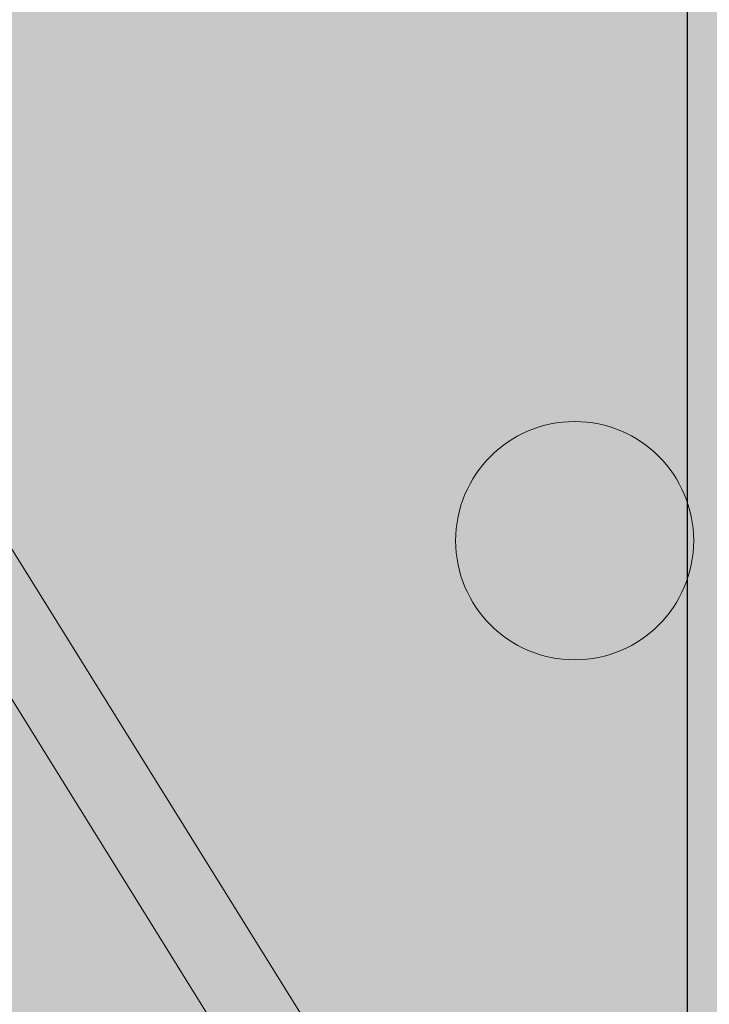
# Model space of a CAD drawing. Units: millimetres. Extents: x 11032 to 26788, y 3406 to 24505.
# Tile 52 of 78: x 15924 to 16358, y 15746 to 16366. Entities that reach past the tile are written whole.
import ezdxf

# ---------------------------------------------------------------- set-up
doc = ezdxf.new("R2010")
doc.units = ezdxf.units.MM
doc.header["$MEASUREMENT"] = 0
for name, color, linetype, lineweight in [('A-ANNO-DIMS', 2, 'Continuous', 18), ('A-GLAZ', 250, 'Continuous', 20), ('A-ROOF', 7, 'Continuous', 30), ('E-LITE', 7, 'Continuous', 18), ('E-LITE-PATT', 7, 'Continuous', 13)]:
    doc.layers.add(name, color=color, linetype=linetype, lineweight=lineweight)
doc.layers.add('A-GLAZ-FRAM-PATT', color=250, linetype='Continuous', lineweight=13, true_color=0x262627)
doc.layers.add('A-ROOF-PATT', color=9, linetype='Continuous', lineweight=13, true_color=0xc7c8ca)
doc.styles.get("Standard").update_dxf_attribs({"font": 'arial.ttf'})
doc.dimstyles.get("Standard").update_dxf_attribs({"dimtxt": 150, "dimasz": 100, "dimexe": 10, "dimexo": 5, "dimgap": 5, "dimtad": 0, "dimtih": 1, "dimtoh": 1, "dimdec": 0, "dimzin": 0, "dimdsep": 46, "dimtxsty": 'Standard', "dimcen": 0.09, "dimadec": 0, "dimazin": 0, "dimtfac": 1, "dimtdec": 0, "dimtofl": 0, "dimtmove": 0, "dimatfit": 3, "dimfxl": 1, "dimtolj": 1, "dimtzin": 0, "dimarcsym": 0})

# ---------------------------------------------------------------- blocks, each defined once
blk = doc.blocks.new('RECESSED-LIGHT-150')
blk.add_circle((75, 75), 75)
blk = doc.blocks.new('*D36')
at = {"layer": 'A-ANNO-DIMS', "color": 0, "lineweight": -2, "transparency": 16777216}
for p, q in [((12301.26, 17115.89), (12301.26, 24416.86)), ((25397.4, 4466.4), (25397.4, 24416.86)), ((12401.26, 24406.86), (18569.2, 24406.86)), ((25297.4, 24406.86), (19129.47, 24406.86))]:
    blk.add_line(p, q, dxfattribs=at)
at = {"layer": 'A-ANNO-DIMS', "color": 0, "transparency": 16777216}
for points in [[(12401.26, 24423.52), (12401.26, 24390.19), (12301.26, 24406.86)], [(25297.4, 24423.52), (25297.4, 24390.19), (25397.4, 24406.86)]]:
    blk.add_solid(points, dxfattribs=at)
at = {"layer": 'Defpoints', "color": 0, "transparency": 16777216}
for p in [(25397.4, 24406.86), (12301.26, 17110.89), (25397.4, 4461.4)]:
    blk.add_point(p, dxfattribs=at)
at = {"layer": 'A-ANNO-DIMS', "color": 0, "transparency": 16777216, "insert": (18849.33, 24406.86), "char_height": 150, "attachment_point": 5}
blk.add_mtext('\\A1;13096', dxfattribs=at)
blk = doc.blocks.new('*D37')
at = {"layer": 'A-ANNO-DIMS', "color": 0, "lineweight": -2, "transparency": 16777216}
for p, q in [((18087.74, 23450.36), (11334.76, 23450.36)), ((11344.76, 23350.36), (11344.76, 14037.46)), ((11344.76, 4561.4), (11344.76, 13874.29)), ((12927.66, 4461.4), (11334.76, 4461.4))]:
    blk.add_line(p, q, dxfattribs=at)
at = {"layer": 'A-ANNO-DIMS', "color": 0, "transparency": 16777216}
for points in [[(11328.1, 23350.36), (11361.43, 23350.36), (11344.76, 23450.36)], [(11328.1, 4561.4), (11361.43, 4561.4), (11344.76, 4461.4)]]:
    blk.add_solid(points, dxfattribs=at)
at = {"layer": 'Defpoints', "color": 0, "transparency": 16777216}
for p in [(11344.76, 23450.36), (18092.74, 23450.36), (12932.66, 4461.4)]:
    blk.add_point(p, dxfattribs=at)
at = {"layer": 'A-ANNO-DIMS', "color": 0, "transparency": 16777216, "insert": (11344.76, 13955.88), "char_height": 150, "attachment_point": 5}
blk.add_mtext('\\A1;18989', dxfattribs=at)
blk = doc.blocks.new('*D45')
at = {"layer": 'A-ANNO-DIMS', "color": 0, "lineweight": -2, "transparency": 16777216}
for p, q in [((13792.37, 18518.92), (26363.9, 18518.92)), ((26353.9, 18418.92), (26353.9, 17450.32)), ((26353.9, 16318.44), (26353.9, 17287.05)), ((22902.4, 16218.44), (26363.9, 16218.44))]:
    blk.add_line(p, q, dxfattribs=at)
at = {"layer": 'A-ANNO-DIMS', "color": 0, "transparency": 16777216}
for points in [[(26337.24, 18418.92), (26370.57, 18418.92), (26353.9, 18518.92)], [(26337.24, 16318.44), (26370.57, 16318.44), (26353.9, 16218.44)]]:
    blk.add_solid(points, dxfattribs=at)
at = {"layer": 'Defpoints', "color": 0, "transparency": 16777216}
for p in [(13787.37, 18518.92), (26353.9, 18518.92), (22897.4, 16218.44)]:
    blk.add_point(p, dxfattribs=at)
at = {"layer": 'A-ANNO-DIMS', "color": 0, "transparency": 16777216, "insert": (26353.9, 17368.68), "char_height": 150, "attachment_point": 5}
blk.add_mtext('\\A1;2300.5', dxfattribs=at)
blk = doc.blocks.new('*D57')
at = {"layer": 'A-ANNO-DIMS', "color": 0, "lineweight": -2, "transparency": 16777216}
for p, q in [((14994.7, 7266.4), (14994.7, 24416.86)), ((20894.7, 7266.4), (20894.7, 24416.86)), ((15094.7, 24406.86), (17715.98, 24406.86)), ((20794.7, 24406.86), (18173.42, 24406.86))]:
    blk.add_line(p, q, dxfattribs=at)
at = {"layer": 'A-ANNO-DIMS', "color": 0, "transparency": 16777216}
for points in [[(15094.7, 24423.52), (15094.7, 24390.19), (14994.7, 24406.86)], [(20794.7, 24423.52), (20794.7, 24390.19), (20894.7, 24406.86)]]:
    blk.add_solid(points, dxfattribs=at)
at = {"layer": 'Defpoints', "color": 0, "transparency": 16777216}
for p in [(20894.7, 24406.86), (14994.7, 7261.4), (20894.7, 7261.4)]:
    blk.add_point(p, dxfattribs=at)
at = {"layer": 'A-ANNO-DIMS', "color": 0, "transparency": 16777216, "insert": (17944.7, 24406.86), "char_height": 150, "attachment_point": 5}
blk.add_mtext('\\A1;5900', dxfattribs=at)
blk = doc.blocks.new('*D60')
at = {"layer": 'A-ANNO-DIMS', "color": 0, "lineweight": -2, "transparency": 16777216}
for p, q in [((14994.7, 7266.4), (14994.7, 24416.86)), ((16344.7, 7266.4), (16344.7, 24416.86)), ((15094.7, 24406.86), (15448.04, 24406.86)), ((16244.7, 24406.86), (15891.36, 24406.86))]:
    blk.add_line(p, q, dxfattribs=at)
at = {"layer": 'A-ANNO-DIMS', "color": 0, "transparency": 16777216}
for points in [[(15094.7, 24423.52), (15094.7, 24390.19), (14994.7, 24406.86)], [(16244.7, 24423.52), (16244.7, 24390.19), (16344.7, 24406.86)]]:
    blk.add_solid(points, dxfattribs=at)
at = {"layer": 'Defpoints', "color": 0, "transparency": 16777216}
for p in [(16344.7, 24406.86), (14994.7, 7261.4), (16344.7, 7261.4)]:
    blk.add_point(p, dxfattribs=at)
at = {"layer": 'A-ANNO-DIMS', "color": 0, "transparency": 16777216, "insert": (15669.7, 24406.86), "char_height": 150, "attachment_point": 5}
blk.add_mtext('\\A1;1350', dxfattribs=at)

msp = doc.modelspace()

# ---------------------------------------------------------------- hatches: boundary and pattern name
at = {"layer": 'A-GLAZ-FRAM-PATT'}
h = msp.add_hatch(color=256, dxfattribs=at)
edge = h.paths.add_edge_path()
edge.add_line((15784.393, 16248.213), (15784.393, 16153.61))
edge.add_line((15784.393, 16153.61), (16560.042, 14907.752))
edge.add_spline(control_points=[(16560.042, 14907.752), (16569.192, 14907.664), (16578.343, 14907.575), (16587.493, 14907.486), (16598.103, 14907.383), (16608.713, 14907.281), (16619.296, 14907.181)], knot_values=[1012.2878735, 1012.2878735, 1012.2878735, 1012.2878735, 1027.155312, 1027.155312, 1027.155312, 1044.3939449, 1044.3939449, 1044.3939449, 1044.3939449], degree=3, periodic=0)
edge.add_line((16619.296, 14907.181), (15784.393, 16248.213))
at = {"layer": 'A-ROOF-PATT'}
h = msp.add_hatch(color=256, dxfattribs=at)
edge = h.paths.add_edge_path()
edge.add_spline(control_points=[(17532.827, 17324.837), (17391.335, 17349.016), (16840.872, 17494.912), (16080.055, 18069.544), (14738.803, 18299.641), (13382.429, 18838.336), (12580.532, 17870.207), (12430.422, 17563.822)], knot_values=[2977.6027945, 2977.6027945, 2977.6027945, 2977.6027945, 3438.1840601, 4811.6463022, 5622.8675483, 7588.0288188, 8560.6685791, 8560.6685791, 8560.6685791, 8560.6685791], degree=3, periodic=0)
edge.add_spline(control_points=[(12430.422, 17563.822), (12437.904, 17573.36), (12445.386, 17582.899), (12452.869, 17592.437), (12452.869, 17592.438), (12452.869, 17592.438), (12452.869, 17592.438)], knot_values=[1408.564138, 1408.564138, 1408.564138, 1408.564138, 1444.85989, 1444.85989, 1444.85989, 1444.8601183, 1444.8601183, 1444.8601183, 1444.8601183], degree=3, periodic=0)
edge.add_spline(control_points=[(12452.869, 17592.438), (12555.432, 17723.185), (12736.557, 17929.686), (13044.86, 18114.643), (13219.943, 18189.644), (13299.92, 18220.646)], knot_values=[339.318246, 339.318246, 339.318246, 339.318246, 836.8349967, 1151.2512933, 1408.564138, 1408.564138, 1408.564138, 1408.564138], degree=3, periodic=0)
edge.add_spline(control_points=[(13299.92, 18220.646), (13299.998, 18220.689), (13300.077, 18220.732), (13319.738, 18231.488), (13339.24, 18241.402), (13388.645, 18264.703), (13418.466, 18277.069), (13478.019, 18298.648), (13507.751, 18307.861), (13544.561, 18317.488), (13551.584, 18319.245), (13558.612, 18320.924)], knot_values=[3783.8950972, 3783.8950972, 3783.8950972, 3783.8950972, 3784.1737101, 3784.1737101, 3853.4666747, 3853.4666747, 3960.2401917, 3960.2401917, 4067.0137087, 4067.0137087, 4092.1744649, 4092.1744649, 4092.1744649, 4092.1744649], degree=3, periodic=0)
edge.add_spline(control_points=[(13558.612, 18320.924), (13581.407, 18326.373), (13604.25, 18331.007), (13657.184, 18339.957), (13687.338, 18343.732), (13748.098, 18348.892), (13778.704, 18350.276), (13840.46, 18350.833), (13871.609, 18350.005), (13934.496, 18346.313), (13966.232, 18343.449), (14030.297, 18335.871), (14062.625, 18331.158), (14127.853, 18320.088), (14160.753, 18313.73), (14241.357, 18296.556), (14289.343, 18284.997), (14386.31, 18259.688), (14435.291, 18245.941), (14534.161, 18217.034), (14584.049, 18201.875), (14684.682, 18170.964), (14735.427, 18155.212), (14837.763, 18123.971), (14889.354, 18108.482), (14954.971, 18089.677), (14968.586, 18085.823), (14992.391, 18079.184), (15002.566, 18076.376), (15021.739, 18071.153), (15030.731, 18068.729), (15047.707, 18064.21), (15055.694, 18062.106), (15079.815, 18055.825), (15095.905, 18051.728), (15143.966, 18039.717), (15175.729, 18032.084), (15254.84, 18013.501), (15301.798, 18002.866), (15394.186, 17981.845), (15439.615, 17971.459), (15528.833, 17950.135), (15572.62, 17939.197), (15658.477, 17916.021), (15700.546, 17903.785), (15753.633, 17886.734), (15765.446, 17882.835), (15786.574, 17875.653), (15795.915, 17872.404), (15810.108, 17867.349), (15814.99, 17865.588), (15824.736, 17862.029), (15829.611, 17860.226), (15844.241, 17854.75), (15854.002, 17851.008), (15883.312, 17839.521), (15902.885, 17831.512), (15966.355, 17804.548), (16010.39, 17784.302), (16098.838, 17741.267), (16143.25, 17718.478), (16232.497, 17671.098), (16277.332, 17646.507), (16367.515, 17596.295), (16412.862, 17570.676), (16504.202, 17519.209), (16550.194, 17493.362), (16643.009, 17442.263), (16689.831, 17417.011), (16756.517, 17382.472), (16775.937, 17372.58), (16795.455, 17362.84)], knot_values=[4092.1744649, 4092.1744649, 4092.1744649, 4092.1744649, 4173.7872258, 4173.7872258, 4280.5607428, 4280.5607428, 4387.3342598, 4387.3342598, 4494.1077768, 4494.1077768, 4600.8812939, 4600.8812939, 4707.6548109, 4707.6548109, 4814.4283279, 4814.4283279, 4967.1262405, 4967.1262405, 5119.8241531, 5119.8241531, 5272.5220657, 5272.5220657, 5425.2199783, 5425.2199783, 5577.9178908, 5577.9178908, 5617.7853319, 5617.7853319, 5647.4648479, 5647.4648479, 5673.611025, 5673.611025, 5696.747607, 5696.747607, 5743.6818903, 5743.6818903, 5837.5504571, 5837.5504571, 5979.7261046, 5979.7261046, 6121.9017521, 6121.9017521, 6264.0773996, 6264.0773996, 6406.2530471, 6406.2530471, 6447.2585849, 6447.2585849, 6480.0420882, 6480.0420882, 6497.3077062, 6497.3077062, 6514.5733242, 6514.5733242, 6549.1045602, 6549.1045602, 6618.1670322, 6618.1670322, 6772.6610171, 6772.6610171, 6927.155002, 6927.155002, 7081.6489869, 7081.6489869, 7236.1429718, 7236.1429718, 7390.6369567, 7390.6369567, 7545.1309416, 7545.1309416, 7608.1992868, 7608.1992868, 7608.1992868, 7608.1992868], degree=3, periodic=0)
edge.add_spline(control_points=[(16795.455, 17362.84), (16814.335, 17349.456), (16832.897, 17336.263), (16873.225, 17307.197), (16894.778, 17291.386), (16936.221, 17259.941), (16956.11, 17244.308), (16993.863, 17213.094), (17011.726, 17197.514), (17041.993, 17169.265), (17054.791, 17156.601), (17078.762, 17131.225), (17089.933, 17118.516), (17110.618, 17092.991), (17120.131, 17080.178), (17130.17, 17065.264), (17131.487, 17063.277), (17133.77, 17059.776), (17134.746, 17058.261), (17136.69, 17055.205), (17137.657, 17053.668), (17140.539, 17049.025), (17142.438, 17045.89), (17148.068, 17036.367), (17151.732, 17029.859), (17163.03, 17008.788), (17170.335, 16993.646), (17184.087, 16961.978), (17190.534, 16945.453), (17202.562, 16911.165), (17208.142, 16893.402), (17218.448, 16856.821), (17223.173, 16838.003), (17231.801, 16799.51), (17235.705, 16779.837), (17241.533, 16746.739), (17243.676, 16733.5), (17247.718, 16706.37), (17249.608, 16692.472), (17252.066, 16672.69), (17252.761, 16666.875), (17254.1, 16655.226), (17254.744, 16649.4), (17256.596, 16631.917), (17257.727, 16620.254), (17260.823, 16585.238), (17262.489, 16561.858), (17266.551, 16488.654), (17267.658, 16438.661), (17267.349, 16375.228), (17267.193, 16362.07), (17266.95, 16348.891)], knot_values=[15.1130472, 15.1130472, 15.1130472, 15.1130472, 82.6995146, 82.6995146, 165.3990291, 165.3990291, 248.0985437, 248.0985437, 330.7980583, 330.7980583, 397.9419458, 397.9419458, 465.0858333, 465.0858333, 532.2297209, 532.2297209, 542.533741, 542.533741, 550.3568158, 550.3568158, 558.1798906, 558.1798906, 573.8260402, 573.8260402, 605.1183395, 605.1183395, 672.7640614, 672.7640614, 740.4097834, 740.4097834, 808.0555054, 808.0555054, 875.7012273, 875.7012273, 943.3469493, 943.3469493, 987.6613492, 987.6613492, 1033.4121612, 1033.4121612, 1052.3850876, 1052.3850876, 1071.358014, 1071.358014, 1109.3038668, 1109.3038668, 1185.1955724, 1185.1955724, 1346.4419026, 1346.4419026, 1388.5586631, 1388.5586631, 1388.5586631, 1388.5586631], degree=3, periodic=0)
edge.add_spline(control_points=[(17266.95, 16348.891), (17266.95, 16348.891), (17266.95, 16348.891), (17266.95, 16348.891), (17253.182, 15602.417), (17239.414, 14855.943), (17225.646, 14109.469)], knot_values=[1388.5586631, 1388.5586631, 1388.5586631, 1388.5586631, 1388.5589654, 1388.5589654, 1388.5589654, 3774.0767661, 3774.0767661, 3774.0767661, 3774.0767661], degree=3, periodic=0)
edge.add_spline(control_points=[(17225.646, 14109.469), (17226.198, 14109.827), (17226.748, 14110.185), (17242.065, 14120.191), (17255.956, 14130.116), (17274.422, 14144.286), (17279.609, 14148.386), (17284.686, 14152.511)], knot_values=[1926.3423968, 1926.3423968, 1926.3423968, 1926.3423968, 1927.316729, 1927.316729, 1953.5121761, 1953.5121761, 1964.0732348, 1964.0732348, 1964.0732348, 1964.0732348], degree=3, periodic=0)
edge.add_spline(control_points=[(17284.686, 14152.511), (17315.791, 14194.761), (17384.413, 14446.273), (17407.128, 14793.401), (17407.093, 15295.84), (17423.274, 15626.362), (17415.601, 15782.507)], knot_values=[0, 0, 0, 0, 163.2554674, 619.2296767, 1171.8624483, 1621.6355562, 1621.6355562, 1621.6355562, 1621.6355562], degree=3, periodic=0)
edge.add_spline(control_points=[(17415.601, 15782.507), (17438.21, 16077.57), (17410.495, 16533.484), (17390.893, 17030.649), (17301.082, 17169.349)], knot_values=[543.9784753, 543.9784753, 543.9784753, 543.9784753, 1452.9852767, 1960.0114926, 1960.0114926, 1960.0114926, 1960.0114926], degree=3, periodic=0)
edge.add_spline(control_points=[(17301.082, 17169.349), (17346.58, 17157.64), (17392.235, 17147.336), (17467.161, 17132.609), (17496.336, 17127.412), (17525.58, 17122.709)], knot_values=[8131.593939, 8131.593939, 8131.593939, 8131.593939, 8269.7349273, 8269.7349273, 8357.5016646, 8357.5016646, 8357.5016646, 8357.5016646], degree=3, periodic=0)
edge.add_line((17525.58, 17122.709), (17532.827, 17324.837))
edge = h.paths.add_edge_path(flags=17)
edge.add_spline(control_points=[(13340.537, 14602.706), (13316.172, 14726.456), (13323.666, 14932.342), (13637.836, 15081.117), (13863.248, 15171.051), (14002.1, 15224.503), (14058.539, 15244.876)], knot_values=[680.8931862, 680.8931862, 680.8931862, 680.8931862, 1033.4728289, 1337.4008326, 1604.7214264, 1784.2944722, 1784.2944722, 1784.2944722, 1784.2944722], degree=3, periodic=0)
edge.add_spline(control_points=[(14058.539, 15244.876), (14058.289, 15275.236), (14057.634, 15305.434), (14055.312, 15376.527), (14053.359, 15417.248), (14048.642, 15497.048), (14045.89, 15536.143), (14042.888, 15574.619)], knot_values=[6573.1065419, 6573.1065419, 6573.1065419, 6573.1065419, 6636.7330012, 6636.7330012, 6723.8890547, 6723.8890547, 6809.6328771, 6809.6328771, 6809.6328771, 6809.6328771], degree=3, periodic=0)
edge.add_spline(control_points=[(14042.888, 15574.619), (13546.54, 15403.221), (13074.735, 15143.241), (13277.36, 14695.339), (13340.537, 14602.706)], knot_values=[503.7925783, 503.7925783, 503.7925783, 503.7925783, 1728.1787606, 2051.34844, 2051.34844, 2051.34844, 2051.34844], degree=3, periodic=0)
h = msp.add_hatch(color=256, dxfattribs=at)
h.set_gradient(color1=(254, 234, 185), color2=(254, 204, 102), name='HEMISPHERICAL')
edge = h.paths.add_edge_path()
edge.add_line((15084.393, 17001.32), (15284.393, 17051.32))
edge.add_line((15284.393, 17051.32), (15470.537, 16752.334))
edge.add_spline(control_points=[(15470.537, 16752.334), (15683.311, 16831.508), (16106.827, 16912.335), (16625.609, 16876.997), (17083.498, 16357.78), (17257.801, 16180.113)], knot_values=[0, 0, 0, 0, 655.2936334, 1252.0157838, 1989.6162859, 1989.6162859, 1989.6162859, 1989.6162859], degree=3, periodic=0)
edge.add_spline(control_points=[(17257.801, 16180.113), (17260.851, 16236.372), (17263.9, 16292.632), (17266.95, 16348.891)], knot_values=[1132.9967717, 1132.9967717, 1132.9967717, 1132.9967717, 1198.0464225, 1198.0464225, 1198.0464225, 1198.0464225], degree=3, periodic=0)
edge.add_spline(control_points=[(17266.95, 16348.891), (17267.193, 16362.07), (17267.349, 16375.228), (17267.658, 16438.661), (17266.551, 16488.654), (17262.489, 16561.858), (17260.823, 16585.238), (17257.727, 16620.254), (17256.596, 16631.917), (17254.744, 16649.4), (17254.1, 16655.226), (17252.761, 16666.875), (17252.066, 16672.69), (17249.608, 16692.472), (17247.718, 16706.37), (17243.676, 16733.5), (17241.533, 16746.739), (17235.705, 16779.837), (17231.801, 16799.51), (17223.173, 16838.003), (17218.448, 16856.821), (17208.142, 16893.402), (17202.562, 16911.165), (17190.534, 16945.453), (17184.087, 16961.978), (17170.335, 16993.646), (17163.03, 17008.788), (17151.732, 17029.859), (17148.068, 17036.367), (17142.438, 17045.89), (17140.539, 17049.025), (17137.657, 17053.668), (17136.69, 17055.205), (17134.746, 17058.261), (17133.77, 17059.776), (17131.487, 17063.277), (17130.17, 17065.264), (17120.131, 17080.178), (17110.618, 17092.991), (17089.933, 17118.516), (17078.762, 17131.225), (17054.791, 17156.601), (17041.993, 17169.265), (17011.726, 17197.514), (16993.863, 17213.094), (16956.11, 17244.308), (16936.221, 17259.941), (16894.778, 17291.386), (16873.225, 17307.197), (16832.897, 17336.263), (16814.335, 17349.456), (16795.455, 17362.84)], knot_values=[15.1130472, 15.1130472, 15.1130472, 15.1130472, 57.2298077, 57.2298077, 218.4761379, 218.4761379, 294.3678435, 294.3678435, 332.3136963, 332.3136963, 351.2866227, 351.2866227, 370.2595491, 370.2595491, 416.0103612, 416.0103612, 460.324761, 460.324761, 527.970483, 527.970483, 595.616205, 595.616205, 663.2619269, 663.2619269, 730.9076489, 730.9076489, 798.5533709, 798.5533709, 829.8456701, 829.8456701, 845.4918197, 845.4918197, 853.3148945, 853.3148945, 861.1379693, 861.1379693, 871.4419895, 871.4419895, 938.585877, 938.585877, 1005.7297645, 1005.7297645, 1072.8736521, 1072.8736521, 1155.5731666, 1155.5731666, 1238.2726812, 1238.2726812, 1320.9721958, 1320.9721958, 1388.5586631, 1388.5586631, 1388.5586631, 1388.5586631], degree=3, periodic=0)
edge.add_spline(control_points=[(16795.455, 17362.84), (16775.937, 17372.58), (16756.517, 17382.472), (16689.831, 17417.011), (16643.009, 17442.263), (16550.194, 17493.362), (16504.202, 17519.209), (16412.862, 17570.676), (16367.515, 17596.295), (16277.332, 17646.507), (16232.497, 17671.098), (16143.25, 17718.478), (16098.838, 17741.267), (16010.39, 17784.302), (15966.355, 17804.548), (15902.885, 17831.512), (15883.312, 17839.521), (15854.002, 17851.008), (15844.241, 17854.75), (15829.611, 17860.226), (15824.736, 17862.029), (15814.99, 17865.588), (15810.108, 17867.349), (15795.915, 17872.404), (15786.574, 17875.653), (15765.446, 17882.835), (15753.633, 17886.734), (15700.546, 17903.785), (15658.477, 17916.021), (15572.62, 17939.197), (15528.833, 17950.135), (15439.615, 17971.459), (15394.186, 17981.845), (15301.798, 18002.866), (15254.84, 18013.501), (15175.729, 18032.084), (15143.966, 18039.717), (15095.905, 18051.728), (15079.815, 18055.825), (15055.694, 18062.106), (15047.707, 18064.21), (15030.731, 18068.729), (15021.739, 18071.153), (15002.566, 18076.376), (14992.391, 18079.184), (14968.586, 18085.823), (14954.971, 18089.677), (14889.354, 18108.482), (14837.763, 18123.971), (14735.427, 18155.212), (14684.682, 18170.964), (14584.049, 18201.875), (14534.161, 18217.034), (14435.291, 18245.941), (14386.31, 18259.688), (14289.343, 18284.997), (14241.357, 18296.556), (14160.753, 18313.73), (14127.853, 18320.088), (14062.625, 18331.158), (14030.297, 18335.871), (13966.232, 18343.449), (13934.496, 18346.313), (13871.609, 18350.005), (13840.46, 18350.833), (13778.704, 18350.276), (13748.098, 18348.892), (13687.338, 18343.732), (13657.184, 18339.957), (13604.25, 18331.007), (13581.407, 18326.373), (13558.612, 18320.924)], knot_values=[4092.1744649, 4092.1744649, 4092.1744649, 4092.1744649, 4155.2428101, 4155.2428101, 4309.736795, 4309.736795, 4464.2307799, 4464.2307799, 4618.7247648, 4618.7247648, 4773.2187497, 4773.2187497, 4927.7127346, 4927.7127346, 5082.2067195, 5082.2067195, 5151.2691915, 5151.2691915, 5185.8004275, 5185.8004275, 5203.0660455, 5203.0660455, 5220.3316635, 5220.3316635, 5253.1151668, 5253.1151668, 5294.1207046, 5294.1207046, 5436.2963521, 5436.2963521, 5578.4719996, 5578.4719996, 5720.6476471, 5720.6476471, 5862.8232946, 5862.8232946, 5956.6918614, 5956.6918614, 6003.6261447, 6003.6261447, 6026.7627267, 6026.7627267, 6052.9089038, 6052.9089038, 6082.5884198, 6082.5884198, 6122.4558609, 6122.4558609, 6275.1537734, 6275.1537734, 6427.851686, 6427.851686, 6580.5495986, 6580.5495986, 6733.2475112, 6733.2475112, 6885.9454238, 6885.9454238, 6992.7189408, 6992.7189408, 7099.4924578, 7099.4924578, 7206.2659749, 7206.2659749, 7313.0394919, 7313.0394919, 7419.8130089, 7419.8130089, 7526.5865259, 7526.5865259, 7608.1992868, 7608.1992868, 7608.1992868, 7608.1992868], degree=3, periodic=0)
edge.add_spline(control_points=[(13558.612, 18320.924), (13472.381, 18287.498), (13386.15, 18254.072), (13299.92, 18220.646), (13299.92, 18220.646), (13299.92, 18220.646), (13299.92, 18220.646)], knot_values=[61.8832457, 61.8832457, 61.8832457, 61.8832457, 339.3179746, 339.3179746, 339.3179746, 339.318246, 339.318246, 339.318246, 339.318246], degree=3, periodic=0)
edge.add_spline(control_points=[(13299.92, 18220.646), (13219.943, 18189.644), (13044.86, 18114.643), (12736.557, 17929.686), (12555.432, 17723.185), (12452.869, 17592.438)], knot_values=[339.318246, 339.318246, 339.318246, 339.318246, 596.6310906, 911.0473872, 1408.564138, 1408.564138, 1408.564138, 1408.564138], degree=3, periodic=0)
edge.add_spline(control_points=[(12452.869, 17592.438), (12452.869, 17592.438), (12452.869, 17592.438), (12452.869, 17592.437), (12445.386, 17582.899), (12437.904, 17573.36), (12430.422, 17563.822)], knot_values=[1408.564138, 1408.564138, 1408.564138, 1408.564138, 1408.5643663, 1408.5643663, 1408.5643663, 1444.8601183, 1444.8601183, 1444.8601183, 1444.8601183], degree=3, periodic=0)
edge.add_spline(control_points=[(12430.422, 17563.822), (12373.797, 17448.248), (12157.302, 16836.764), (12751.985, 16393.69), (13424.325, 15907.903), (14042.888, 15574.619)], knot_values=[0, 0, 0, 0, 366.8993034, 1975.5941082, 2977.6027945, 2977.6027945, 2977.6027945, 2977.6027945], degree=3, periodic=0)
edge.add_spline(control_points=[(14042.888, 15574.619), (14042.839, 15575.252), (14042.789, 15575.886), (14039.681, 15615.607), (14036.366, 15654.052), (14029.551, 15729.305), (14026.05, 15766.114), (14019.175, 15837.686), (14015.8, 15872.45), (13903.823, 16338.596)], knot_values=[6310.2261504, 6310.2261504, 6310.2261504, 6310.2261504, 6311.6383814, 6311.6383814, 6398.7944349, 6398.7944349, 6485.9504884, 6485.9504884, 6573.1065419, 6573.1065419, 6573.1065419, 6573.1065419], degree=3, periodic=0)
edge.add_spline(control_points=[(13903.823, 16338.596), (14237.315, 16236.889), (14456.623, 16167.555), (14614.196, 16115.84)], knot_values=[0, 0, 0, 0, 202.9853419, 202.9853419, 202.9853419, 202.9853419], degree=3, periodic=0)
edge.add_spline(control_points=[(14614.196, 16115.84), (14663.209, 16178.992), (14799.965, 16341.237), (14969.915, 16481.426), (15084.393, 16556.825)], knot_values=[2405.0345045, 2405.0345045, 2405.0345045, 2405.0345045, 2644.8826966, 3039.2707272, 3039.2707272, 3039.2707272, 3039.2707272], degree=3, periodic=0)
edge.add_line((15084.393, 16556.825), (15084.393, 17001.32))
h.paths.add_polyline_path([(14195.599, 17606.181, -1), (14395.599, 17606.181, -1)], flags=16)
h.paths.add_polyline_path([(13310.178, 17032.97, -1), (13510.178, 17032.97, -1)], flags=16)
h = msp.add_hatch(color=256, dxfattribs=at)
h.set_gradient(color1=(254, 234, 185), color2=(254, 204, 102), name='HEMISPHERICAL')
edge = h.paths.add_edge_path()
edge.add_spline(control_points=[(16560.042, 14907.752), (16569.192, 14907.664), (16578.343, 14907.575), (16587.493, 14907.486), (16832.101, 14905.115), (17122.895, 14902.296), (16849.359, 14976.117), (16870.954, 15304.114), (17098.337, 15241.178), (17235.385, 15203.245)], knot_values=[0, 0, 0, 0, 14.8674385, 14.8674385, 14.8674385, 412.2943091, 487.3345915, 708.6416004, 1044.3939449, 1044.3939449, 1044.3939449, 1044.3939449], degree=3, periodic=0)
edge.add_line((16587.504, 14907.486), (16560.207, 14907.486))
edge.add_line((16560.207, 14907.486), (15784.393, 16153.61))
edge.add_line((15784.393, 16153.61), (15784.393, 15385.996))
edge.add_spline(control_points=[(15784.393, 15385.996), (15798.391, 15360.52), (15847.198, 15266.214), (15887.196, 15168.614), (15912.903, 15096.727)], knot_values=[1463.2850479, 1463.2850479, 1463.2850479, 1463.2850479, 1550.659771, 1779.9599361, 1779.9599361, 1779.9599361, 1779.9599361], degree=3, periodic=0)
edge.add_spline(control_points=[(15912.903, 15096.727), (15913.652, 15095.649), (15914.403, 15094.565), (15925.191, 15078.948), (15935.516, 15063.47), (15956.582, 15030.918), (15967.324, 15013.844), (15989.119, 14978.386), (16000.173, 14960.003), (16022.525, 14922.193), (16033.824, 14902.767), (16056.63, 14863.116), (16068.138, 14842.891), (16091.349, 14801.871), (16103.053, 14781.075), (16126.666, 14739.118), (16138.575, 14717.958), (16162.628, 14675.459), (16174.772, 14654.12), (16199.352, 14611.428), (16211.787, 14590.075), (16237.037, 14547.491), (16249.851, 14526.26), (16271.946, 14490.566), (16281.092, 14476.044), (16299.694, 14447.129), (16309.149, 14432.737), (16328.456, 14404.098), (16338.307, 14389.85), (16358.518, 14361.503), (16368.879, 14347.403), (16390.266, 14319.347), (16401.291, 14305.391), (16420.626, 14281.969), (16428.703, 14272.467), (16445.363, 14253.527), (16453.946, 14244.088), (16471.727, 14225.278), (16480.926, 14215.907), (16500.075, 14197.247), (16510.026, 14187.959), (16530.844, 14169.504), (16541.71, 14160.337), (16564.549, 14142.195), (16576.522, 14133.22), (16597.69, 14118.448), (16606.528, 14112.565), (16624.87, 14101.004), (16634.376, 14095.326), (16654.117, 14084.255), (16664.352, 14078.862), (16685.603, 14068.46), (16696.619, 14063.452), (16719.46, 14053.944), (16731.285, 14049.444), (16755.742, 14041.097), (16768.374, 14037.251), (16794.396, 14030.368), (16807.787, 14027.332), (16835.229, 14022.23), (16849.279, 14020.163), (16877.882, 14017.141), (16892.435, 14016.186), (16921.835, 14015.489), (16936.683, 14015.749), (16961.564, 14017.241), (16971.582, 14018.127), (16986.57, 14019.883), (16991.56, 14020.54), (16999.027, 14021.63), (17001.514, 14022.011), (17006.48, 14022.809), (17008.962, 14023.225), (17014.824, 14024.251), (17018.193, 14024.875), (17036.262, 14028.398), (17050.55, 14031.826), (17078.171, 14039.583), (17091.505, 14043.912), (17115.643, 14052.705), (17126.557, 14057.089), (17137.108, 14061.688)], knot_values=[2010.7639617, 2010.7639617, 2010.7639617, 2010.7639617, 2014.7029827, 2014.7029827, 2067.238337, 2067.238337, 2119.7736913, 2119.7736913, 2172.3090457, 2172.3090457, 2224.8444, 2224.8444, 2277.3797543, 2277.3797543, 2329.9151086, 2329.9151086, 2382.450463, 2382.450463, 2434.9858173, 2434.9858173, 2487.5211716, 2487.5211716, 2540.0565259, 2540.0565259, 2576.3179289, 2576.3179289, 2612.5793318, 2612.5793318, 2648.8407347, 2648.8407347, 2685.1021376, 2685.1021376, 2721.3635405, 2721.3635405, 2746.252015, 2746.252015, 2771.1404895, 2771.1404895, 2796.028964, 2796.028964, 2820.9174385, 2820.9174385, 2845.8059131, 2845.8059131, 2870.6943876, 2870.6943876, 2887.5132757, 2887.5132757, 2904.3321639, 2904.3321639, 2921.1510521, 2921.1510521, 2937.9699402, 2937.9699402, 2954.7888284, 2954.7888284, 2971.6077166, 2971.6077166, 2988.4266047, 2988.4266047, 3005.2454929, 3005.2454929, 3022.0643811, 3022.0643811, 3038.8832692, 3038.8832692, 3050.1975453, 3050.1975453, 3055.8546833, 3055.8546833, 3058.6832524, 3058.6832524, 3061.5118214, 3061.5118214, 3065.3934173, 3065.3934173, 3082.4668716, 3082.4668716, 3099.5403259, 3099.5403259, 3114.5433443, 3114.5433443, 3114.5433443, 3114.5433443], degree=3, periodic=0)
edge.add_spline(control_points=[(17137.108, 14061.688), (17165.253, 14274.398), (17209.97, 14653.885), (17230.2, 15035.586), (17235.385, 15203.245)], knot_values=[1968.0804557, 1968.0804557, 1968.0804557, 1968.0804557, 2611.5282875, 3114.5379264, 3114.5379264, 3114.5379264, 3114.5379264], degree=3, periodic=0)
edge = h.paths.add_edge_path()
edge.add_spline(control_points=[(16856.103, 14956.992), (16852.841, 14961.219), (16849.83, 14965.576), (16842.539, 14977.287), (16838.658, 14984.798), (16832.033, 15000.109), (16829.289, 15007.911), (16824.126, 15026.008), (16822.047, 15036.354), (16819.308, 15057.097), (16818.649, 15067.496), (16818.576, 15088.188), (16819.162, 15098.483), (16821.467, 15118.823), (16823.186, 15128.868), (16827.696, 15148.567), (16830.486, 15158.22), (16836.065, 15173.969), (16838.565, 15180.211), (16844.079, 15192.402), (16847.092, 15198.353), (16852.029, 15207.021), (16853.744, 15209.868), (16857.321, 15215.468), (16859.188, 15218.226), (16863.017, 15223.558), (16864.978, 15226.136), (16872.565, 15235.558), (16878.593, 15241.952), (16891.428, 15253.591), (16898.232, 15258.834), (16912.397, 15268.127), (16919.756, 15272.176), (16934.816, 15279.138), (16942.515, 15282.052), (16958.1, 15286.873), (16965.985, 15288.78), (16984.013, 15292.142), (16994.186, 15293.334), (17014.631, 15294.619), (17024.904, 15294.713), (17048.453, 15293.935), (17061.76, 15292.783), (17088.519, 15289.422), (17101.972, 15287.211), (17131.961, 15281.46), (17148.526, 15277.734), (17181.692, 15269.627), (17198.292, 15265.245), (17222.182, 15258.759), (17229.535, 15256.737), (17236.862, 15254.714)], knot_values=[9.6639535, 9.6639535, 9.6639535, 9.6639535, 20.0351668, 20.0351668, 36.9411752, 36.9411752, 53.8471837, 53.8471837, 75.7795687, 75.7795687, 97.7119538, 97.7119538, 119.6443388, 119.6443388, 141.5767238, 141.5767238, 163.5091089, 163.5091089, 178.3829945, 178.3829945, 193.2568801, 193.2568801, 200.6938229, 200.6938229, 208.1307657, 208.1307657, 215.4448585, 215.4448585, 235.5795923, 235.5795923, 255.7143261, 255.7143261, 275.8490598, 275.8490598, 295.9837936, 295.9837936, 316.1185274, 316.1185274, 341.7220543, 341.7220543, 367.3255812, 367.3255812, 400.1572431, 400.1572431, 432.988905, 432.988905, 473.0440165, 473.0440165, 513.099128, 513.099128, 530.9692999, 530.9692999, 530.9692999, 530.9692999], degree=3, periodic=0)
edge.add_spline(control_points=[(17236.862, 15254.714), (17240.377, 15387.456), (17242.496, 15609.536), (17239.752, 15831.567), (17250.544, 16044.717)], knot_values=[1250.9818616, 1250.9818616, 1250.9818616, 1250.9818616, 1649.1516581, 1916.613987, 1916.613987, 1916.613987, 1916.613987], degree=3, periodic=0)
edge.add_spline(control_points=[(17250.544, 16044.717), (17229.169, 16066.505), (17207.794, 16088.292), (17186.419, 16110.08), (17186.418, 16110.08), (17186.418, 16110.081), (17186.418, 16110.081)], knot_values=[-88.5185581, -88.5185581, -88.5185581, -88.5185581, -0.0012784, -0.0012784, -0.0012784, 0, 0, 0, 0], degree=3, periodic=0)
edge.add_spline(control_points=[(17186.418, 16110.081), (17169.261, 16127.569), (17151.499, 16145.947), (17114.892, 16184.084), (17096.046, 16203.842), (17057.437, 16244.305), (17037.673, 16265.01), (16997.415, 16306.918), (16976.921, 16328.12), (16927.79, 16378.347), (16898.924, 16407.388), (16840.771, 16464.327), (16811.484, 16492.225), (16758.449, 16540.764), (16734.666, 16561.798), (16687.634, 16601.588), (16664.382, 16620.344), (16624.116, 16650.909), (16606.897, 16663.324), (16583.769, 16678.999), (16577.49, 16683.149), (16567.144, 16689.805), (16563.039, 16692.397), (16550.823, 16699.959), (16542.775, 16704.739), (16526.841, 16713.814), (16518.956, 16718.108), (16495.524, 16730.301), (16480.199, 16737.514), (16449.97, 16750.334), (16435.066, 16755.942), (16405.476, 16765.764), (16390.79, 16769.979), (16361.418, 16777.195), (16346.731, 16780.197), (16317.147, 16785.133), (16302.249, 16787.067), (16272.053, 16789.992), (16256.756, 16790.981), (16225.609, 16792.125), (16209.759, 16792.279), (16177.385, 16791.865), (16160.862, 16791.296), (16136.98, 16790.07), (16129.942, 16789.661), (16118.22, 16788.91), (16113.574, 16788.594), (16103.645, 16787.886), (16098.362, 16787.489), (16087.761, 16786.652), (16082.439, 16786.212), (16066.413, 16784.825), (16055.649, 16783.812), (16023.135, 16780.505), (16001.164, 16777.942), (15934.539, 16769.141), (15889.17, 16761.791), (15797.417, 16743.949), (15751.033, 16733.457), (15645.217, 16705.796), (15585.74, 16687.58), (15526.207, 16666.217), (15525.367, 16665.915), (15524.528, 16665.613)], knot_values=[0, 0, 0, 0, 71.0501454, 71.0501454, 142.1002909, 142.1002909, 213.1504363, 213.1504363, 284.2005818, 284.2005818, 381.323193, 381.323193, 478.4458043, 478.4458043, 557.8219847, 557.8219847, 637.1981651, 637.1981651, 698.3122593, 698.3122593, 721.3971375, 721.3971375, 736.7790891, 736.7790891, 767.5429924, 767.5429924, 798.3068957, 798.3068957, 859.8347022, 859.8347022, 921.3625088, 921.3625088, 982.8903154, 982.8903154, 1044.4181219, 1044.4181219, 1105.9459285, 1105.9459285, 1167.4737351, 1167.4737351, 1229.0015416, 1229.0015416, 1290.5293482, 1290.5293482, 1315.8990035, 1315.8990035, 1332.3812792, 1332.3812792, 1350.9052657, 1350.9052657, 1369.4292522, 1369.4292522, 1406.4772252, 1406.4772252, 1480.5731712, 1480.5731712, 1628.7650633, 1628.7650633, 1776.9569554, 1776.9569554, 1966.3109251, 1966.3109251, 1969.019495, 1969.019495, 1969.019495, 1969.019495], degree=3, periodic=0)
edge.add_line((15524.528, 16665.613), (16587.978, 14957.484))
edge.add_spline(control_points=[(16587.978, 14957.484), (16605.253, 14957.316), (16622.516, 14957.149), (16665.945, 14956.759), (16691.933, 14956.554), (16742.419, 14956.302), (16766.918, 14956.255), (16813.531, 14956.412), (16835.647, 14956.617), (16856.103, 14956.992)], knot_values=[872.2181925, 872.2181925, 872.2181925, 872.2181925, 900.2857301, 900.2857301, 943.3659889, 943.3659889, 986.4462476, 986.4462476, 1029.5265064, 1029.5265064, 1029.5265064, 1029.5265064], degree=3, periodic=0)
h.paths.add_polyline_path([(16474.605, 15622.642, -1), (16624.605, 15622.642, -1)], flags=16)
h.paths.add_polyline_path([(16198.536, 16037.613, -1), (16348.536, 16037.613, -1)], flags=16)
h.paths.add_polyline_path([(16475.717, 16408.125, -1), (16625.717, 16408.125, -1)], flags=16)
at = {"layer": 'E-LITE-PATT'}
h = msp.add_hatch(color=256, dxfattribs=at)
h.paths.add_polyline_path([(13510.178, 17032.97, 1), (13310.178, 17032.97, 1)])
h.paths.add_polyline_path([(14395.599, 17606.181, 1), (14195.599, 17606.181, 1)])
h.paths.add_polyline_path([(16625.717, 16408.125, 1), (16475.717, 16408.125, 1)])
h.paths.add_polyline_path([(16348.536, 16037.613, 1), (16198.536, 16037.613, 1)])
h.paths.add_polyline_path([(16624.605, 15622.642, 1), (16474.605, 15622.642, 1)])
edge = h.paths.add_edge_path()
edge.add_spline(control_points=[(17236.862, 15254.714), (17229.535, 15256.737), (17222.182, 15258.759), (17198.292, 15265.245), (17181.692, 15269.627), (17148.526, 15277.734), (17131.961, 15281.46), (17101.972, 15287.211), (17088.519, 15289.422), (17061.76, 15292.783), (17048.453, 15293.935), (17024.904, 15294.713), (17014.631, 15294.619), (16994.186, 15293.334), (16984.013, 15292.142), (16965.985, 15288.78), (16958.1, 15286.873), (16942.515, 15282.052), (16934.816, 15279.138), (16919.756, 15272.176), (16912.397, 15268.127), (16898.232, 15258.834), (16891.428, 15253.591), (16878.593, 15241.952), (16872.565, 15235.558), (16864.978, 15226.136), (16863.017, 15223.558), (16859.188, 15218.226), (16857.321, 15215.468), (16853.744, 15209.868), (16852.029, 15207.021), (16847.092, 15198.353), (16844.079, 15192.402), (16838.565, 15180.211), (16836.065, 15173.969), (16830.486, 15158.22), (16827.696, 15148.567), (16823.186, 15128.868), (16821.467, 15118.823), (16819.162, 15098.483), (16818.576, 15088.188), (16818.649, 15067.496), (16819.308, 15057.097), (16822.047, 15036.354), (16824.126, 15026.008), (16829.289, 15007.911), (16832.033, 15000.109), (16838.658, 14984.798), (16842.539, 14977.287), (16849.83, 14965.576), (16852.841, 14961.219), (16856.103, 14956.992)], knot_values=[9.6639535, 9.6639535, 9.6639535, 9.6639535, 27.5341253, 27.5341253, 67.5892368, 67.5892368, 107.6443483, 107.6443483, 140.4760102, 140.4760102, 173.3076721, 173.3076721, 198.911199, 198.911199, 224.5147259, 224.5147259, 244.6494597, 244.6494597, 264.7841935, 264.7841935, 284.9189272, 284.9189272, 305.053661, 305.053661, 325.1883948, 325.1883948, 332.5024876, 332.5024876, 339.9394304, 339.9394304, 347.3763732, 347.3763732, 362.2502588, 362.2502588, 377.1241444, 377.1241444, 399.0565295, 399.0565295, 420.9889145, 420.9889145, 442.9212995, 442.9212995, 464.8536846, 464.8536846, 486.7860696, 486.7860696, 503.6920781, 503.6920781, 520.5980866, 520.5980866, 530.9692999, 530.9692999, 530.9692999, 530.9692999], degree=3, periodic=0)
edge.add_spline(control_points=[(16856.103, 14956.992), (16835.647, 14956.617), (16813.531, 14956.412), (16766.918, 14956.255), (16742.419, 14956.302), (16691.933, 14956.554), (16665.945, 14956.759), (16622.516, 14957.149), (16605.253, 14957.316), (16587.978, 14957.484)], knot_values=[872.2181925, 872.2181925, 872.2181925, 872.2181925, 915.2984513, 915.2984513, 958.37871, 958.37871, 1001.4589687, 1001.4589687, 1029.5265064, 1029.5265064, 1029.5265064, 1029.5265064], degree=3, periodic=0)
edge.add_line((16587.978, 14957.484), (16619.296, 14907.181))
edge.add_spline(control_points=[(16619.296, 14907.181), (16852.686, 14904.98), (17116.098, 14904.13), (16849.359, 14976.117), (16870.954, 15304.114), (17098.337, 15241.178), (17235.385, 15203.245)], knot_values=[0, 0, 0, 0, 380.1882376, 455.2285201, 676.535529, 1012.2878735, 1012.2878735, 1012.2878735, 1012.2878735], degree=3, periodic=0)
edge.add_spline(control_points=[(17235.385, 15203.245), (17235.916, 15220.399), (17236.408, 15237.556), (17236.862, 15254.714)], knot_values=[1916.613987, 1916.613987, 1916.613987, 1916.613987, 1968.0804557, 1968.0804557, 1968.0804557, 1968.0804557], degree=3, periodic=0)
h = msp.add_hatch(color=256, dxfattribs=at)
h.paths.add_polyline_path([(13510.178, 17032.97, 1), (13310.178, 17032.97, 1)])
h.paths.add_polyline_path([(14195.599, 17606.181, 1), (14395.599, 17606.181, 1)])
h.paths.add_polyline_path([(16625.717, 16408.125, 1), (16475.717, 16408.125, 1)])
h.paths.add_polyline_path([(16198.536, 16037.613, 1), (16348.536, 16037.613, 1)])
h.paths.add_polyline_path([(16474.605, 15622.642, 1), (16624.605, 15622.642, 1)])
h = msp.add_hatch(color=256, dxfattribs=at)
edge = h.paths.add_edge_path()
edge.add_spline(control_points=[(15084.393, 16556.825), (14969.915, 16481.426), (14799.965, 16341.237), (14663.209, 16178.992), (14614.196, 16115.84)], knot_values=[2405.0345045, 2405.0345045, 2405.0345045, 2405.0345045, 2799.422535, 3039.2707272, 3039.2707272, 3039.2707272, 3039.2707272], degree=3, periodic=0)
edge.add_spline(control_points=[(14614.196, 16115.84), (14650.957, 16103.776), (14684.357, 16092.67), (14715.064, 16082.336)], knot_values=[202.9853419, 202.9853419, 202.9853419, 202.9853419, 250.3408615, 250.3408615, 250.3408615, 250.3408615], degree=3, periodic=0)
edge.add_spline(control_points=[(14715.064, 16082.336), (14732.32, 16103.979), (14749.873, 16125.274), (14780.086, 16160.475), (14792.544, 16174.592), (14817.876, 16202.424), (14830.748, 16216.137), (14853.903, 16239.975), (14864.109, 16250.213), (14884.415, 16270.066), (14894.503, 16279.688), (14918.667, 16302.183), (14932.865, 16314.967), (14987.375, 16362.454), (15029.339, 16395.81), (15076.718, 16430.13), (15080.55, 16432.882), (15084.393, 16435.621)], knot_values=[2472.5855096, 2472.5855096, 2472.5855096, 2472.5855096, 2558.786533, 2558.786533, 2617.7975153, 2617.7975153, 2676.8084975, 2676.8084975, 2721.9976237, 2721.9976237, 2765.3424393, 2765.3424393, 2824.4059302, 2824.4059302, 2988.2351723, 2988.2351723, 3002.5987883, 3002.5987883, 3002.5987883, 3002.5987883], degree=3, periodic=0)
edge.add_line((15084.393, 16435.621), (15084.393, 16556.825))
edge = h.paths.add_edge_path()
edge.add_spline(control_points=[(17257.801, 16180.113), (17083.498, 16357.78), (16625.609, 16876.997), (16106.827, 16912.335), (15683.311, 16831.508), (15470.537, 16752.334)], knot_values=[0, 0, 0, 0, 737.600502, 1334.3226525, 1989.6162859, 1989.6162859, 1989.6162859, 1989.6162859], degree=3, periodic=0)
edge.add_line((15470.537, 16752.334), (15524.528, 16665.613))
edge.add_spline(control_points=[(15524.528, 16665.613), (15525.367, 16665.915), (15526.207, 16666.217), (15585.74, 16687.58), (15645.217, 16705.796), (15751.033, 16733.457), (15797.417, 16743.949), (15889.17, 16761.791), (15934.539, 16769.141), (16001.164, 16777.942), (16023.135, 16780.505), (16055.649, 16783.812), (16066.413, 16784.825), (16082.439, 16786.212), (16087.761, 16786.652), (16098.362, 16787.489), (16103.645, 16787.886), (16113.574, 16788.594), (16118.22, 16788.91), (16129.942, 16789.661), (16136.98, 16790.07), (16160.862, 16791.296), (16177.385, 16791.865), (16209.759, 16792.279), (16225.609, 16792.125), (16256.756, 16790.981), (16272.053, 16789.992), (16302.249, 16787.067), (16317.147, 16785.133), (16346.731, 16780.197), (16361.418, 16777.195), (16390.79, 16769.979), (16405.476, 16765.764), (16435.066, 16755.942), (16449.97, 16750.334), (16480.199, 16737.514), (16495.524, 16730.301), (16518.956, 16718.108), (16526.841, 16713.814), (16542.775, 16704.739), (16550.823, 16699.959), (16563.039, 16692.397), (16567.144, 16689.805), (16577.49, 16683.149), (16583.769, 16678.999), (16606.897, 16663.324), (16624.116, 16650.909), (16664.382, 16620.344), (16687.634, 16601.588), (16734.666, 16561.798), (16758.449, 16540.764), (16811.484, 16492.225), (16840.771, 16464.327), (16898.924, 16407.388), (16927.79, 16378.347), (16976.921, 16328.12), (16997.415, 16306.918), (17037.673, 16265.01), (17057.437, 16244.305), (17096.046, 16203.842), (17114.892, 16184.084), (17151.499, 16145.947), (17169.261, 16127.569), (17186.418, 16110.081)], knot_values=[0, 0, 0, 0, 2.7085699, 2.7085699, 192.0625397, 192.0625397, 340.2544317, 340.2544317, 488.4463238, 488.4463238, 562.5422698, 562.5422698, 599.5902428, 599.5902428, 618.1142294, 618.1142294, 636.6382159, 636.6382159, 653.1204915, 653.1204915, 678.4901469, 678.4901469, 740.0179534, 740.0179534, 801.54576, 801.54576, 863.0735665, 863.0735665, 924.6013731, 924.6013731, 986.1291797, 986.1291797, 1047.6569862, 1047.6569862, 1109.1847928, 1109.1847928, 1170.7125993, 1170.7125993, 1201.4765026, 1201.4765026, 1232.2404059, 1232.2404059, 1247.6223576, 1247.6223576, 1270.7072358, 1270.7072358, 1331.8213299, 1331.8213299, 1411.1975103, 1411.1975103, 1490.5736908, 1490.5736908, 1587.696302, 1587.696302, 1684.8189133, 1684.8189133, 1755.8690587, 1755.8690587, 1826.9192041, 1826.9192041, 1897.9693496, 1897.9693496, 1969.019495, 1969.019495, 1969.019495, 1969.019495], degree=3, periodic=0)
edge.add_spline(control_points=[(17186.418, 16110.081), (17186.418, 16110.081), (17186.418, 16110.08), (17186.419, 16110.08), (17207.794, 16088.292), (17229.169, 16066.505), (17250.544, 16044.717)], knot_values=[-88.5185581, -88.5185581, -88.5185581, -88.5185581, -88.5172797, -88.5172797, -88.5172797, 0, 0, 0, 0], degree=3, periodic=0)
edge.add_spline(control_points=[(17250.544, 16044.717), (17251.307, 16059.803), (17252.131, 16075.51), (17253.018, 16091.882)], knot_values=[1232.05171, 1232.05171, 1232.05171, 1232.05171, 1250.9818616, 1250.9818616, 1250.9818616, 1250.9818616], degree=3, periodic=0)
edge.add_spline(control_points=[(17253.018, 16091.882), (17253.019, 16091.892), (17253.019, 16091.901), (17253.02, 16091.911), (17254.614, 16121.312), (17256.207, 16150.712), (17257.801, 16180.113)], knot_values=[1198.0464225, 1198.0464225, 1198.0464225, 1198.0464225, 1198.0576047, 1198.0576047, 1198.0576047, 1232.05171, 1232.05171, 1232.05171, 1232.05171], degree=3, periodic=0)

# ---------------------------------------------------------------- linework, layer by layer
at = {"layer": 'A-GLAZ'}
for p, q in [((15284.393, 17051.32), (16619.296, 14907.181)), ((15284.393, 16956.717), (16560.207, 14907.486))]:
    msp.add_line(p, q, dxfattribs=at)
at = {"layer": 'A-ROOF'}
msp.add_open_spline([(14042.888, 15574.619), (13424.325, 15907.903), (12751.985, 16393.69), (11963.048, 16981.495), (13249.687, 18891.056), (14738.803, 18299.641), (16080.055, 18069.544), (16966.203, 17400.251), (17654.208, 17293.942), (17944.704, 17286.735)], degree=3, knots=[0, 0, 0, 0, 1002.0086862, 2610.7034911, 3950.2425548, 5915.4038253, 6726.6250714, 8100.0873135, 8996.4318779, 8996.4318779, 8996.4318779, 8996.4318779], dxfattribs=at)
at = {"layer": 'E-LITE'}
for points, knots in [([(17257.801, 16180.113), (17083.498, 16357.78), (16625.609, 16876.997), (16069.956, 16914.847), (15586.409, 16811.936), (15334.393, 16695.842)], [0, 0, 0, 0, 737.600502, 1334.3226525, 2131.0201637, 2131.0201637, 2131.0201637, 2131.0201637]), ([(17250.544, 16044.717), (17229.169, 16066.505), (17207.794, 16088.292), (17186.419, 16110.08), (17186.418, 16110.08), (17186.418, 16110.081), (17186.418, 16110.081), (17169.261, 16127.569), (17151.499, 16145.947), (17114.892, 16184.084), (17096.046, 16203.842), (17057.437, 16244.305), (17037.673, 16265.01), (16997.415, 16306.918), (16976.921, 16328.12), (16927.79, 16378.347), (16898.924, 16407.388), (16840.771, 16464.327), (16811.484, 16492.225), (16758.449, 16540.764), (16734.666, 16561.798), (16687.634, 16601.588), (16664.382, 16620.344), (16624.116, 16650.909), (16606.897, 16663.324), (16583.769, 16678.999), (16577.49, 16683.149), (16567.144, 16689.805), (16563.039, 16692.397), (16550.823, 16699.959), (16542.775, 16704.739), (16526.841, 16713.814), (16518.956, 16718.108), (16495.524, 16730.301), (16480.199, 16737.514), (16449.97, 16750.334), (16435.066, 16755.942), (16405.476, 16765.764), (16390.79, 16769.979), (16361.418, 16777.195), (16346.731, 16780.197), (16317.147, 16785.133), (16302.249, 16787.067), (16272.053, 16789.992), (16256.756, 16790.981), (16225.609, 16792.125), (16209.759, 16792.279), (16177.385, 16791.865), (16160.862, 16791.296), (16136.98, 16790.07), (16129.942, 16789.661), (16118.22, 16788.91), (16113.574, 16788.594), (16103.645, 16787.886), (16098.362, 16787.489), (16087.761, 16786.652), (16082.439, 16786.212), (16066.413, 16784.825), (16055.649, 16783.812), (16023.135, 16780.505), (16001.164, 16777.942), (15934.539, 16769.141), (15889.17, 16761.791), (15797.417, 16743.949), (15751.033, 16733.457), (15645.217, 16705.796), (15585.74, 16687.58), (15526.207, 16666.217), (15525.367, 16665.915), (15524.528, 16665.613)], [-88.5185581, -88.5185581, -88.5185581, -88.5185581, -0.0012784, -0.0012784, -0.0012784, 0, 0, 0, 71.0501454, 71.0501454, 142.1002909, 142.1002909, 213.1504363, 213.1504363, 284.2005818, 284.2005818, 381.323193, 381.323193, 478.4458043, 478.4458043, 557.8219847, 557.8219847, 637.1981651, 637.1981651, 698.3122593, 698.3122593, 721.3971375, 721.3971375, 736.7790891, 736.7790891, 767.5429924, 767.5429924, 798.3068957, 798.3068957, 859.8347022, 859.8347022, 921.3625088, 921.3625088, 982.8903154, 982.8903154, 1044.4181219, 1044.4181219, 1105.9459285, 1105.9459285, 1167.4737351, 1167.4737351, 1229.0015416, 1229.0015416, 1290.5293482, 1290.5293482, 1315.8990035, 1315.8990035, 1332.3812792, 1332.3812792, 1350.9052657, 1350.9052657, 1369.4292522, 1369.4292522, 1406.4772252, 1406.4772252, 1480.5731712, 1480.5731712, 1628.7650633, 1628.7650633, 1776.9569554, 1776.9569554, 1966.3109251, 1966.3109251, 1969.019495, 1969.019495, 1969.019495, 1969.019495])]:
    msp.add_open_spline(points, degree=3, knots=knots, dxfattribs=at)

# ---------------------------------------------------------------- block references
msp.add_blockref('RECESSED-LIGHT-150', (16198.536, 15962.613), dxfattribs=at)

# ---------------------------------------------------------------- dimensions: what is measured, and where the dimension line sits
at = {"layer": 'A-ANNO-DIMS'}
for base, p1, p2, picture, middle in [((25397.404, 24406.858), (12301.265, 17110.885), (25397.404, 4461.399), '*D36', (18849.334, 24406.858)), ((20894.704, 24406.858), (14994.704, 7261.399), (20894.704, 7261.399), '*D57', (17944.704, 24406.858)), ((16344.704, 24406.858), (14994.704, 7261.399), (16344.704, 7261.399), '*D60', (15669.704, 24406.858))]:
    dim = msp.add_linear_dim(base=base, p1=p1, p2=p2, dimstyle='Standard', override={"dimdec": 0, "dimlfac": 1, "dimrnd": 0, "dimzin": 0, "dimdsep": 46, "dimlunit": 2}, dxfattribs=at)
    dim.commit()
    dim.dimension.update_dxf_attribs({"geometry": picture, "text_midpoint": middle})
for base, p1, p2, override, picture, middle in [((11344.765, 23450.358), (12932.665, 4461.399), (18092.739, 23450.358), {"dimdec": 0, "dimlfac": 1, "dimrnd": 0, "dimzin": 0, "dimdsep": 46, "dimlunit": 2}, '*D37', (11344.765, 13955.879)), ((26353.904, 18518.925), (22897.404, 16218.44), (13787.367, 18518.925), {"dimdec": 1, "dimlfac": 1, "dimrnd": 0, "dimzin": 0, "dimdsep": 46, "dimlunit": 2}, '*D45', (26353.904, 17368.682))]:
    dim = msp.add_linear_dim(base=base, p1=p1, p2=p2, angle=90, dimstyle='Standard', override=override, dxfattribs=at)
    dim.commit()
    dim.dimension.update_dxf_attribs({"geometry": picture, "text_midpoint": middle})

doc.saveas('drawing.dxf')
